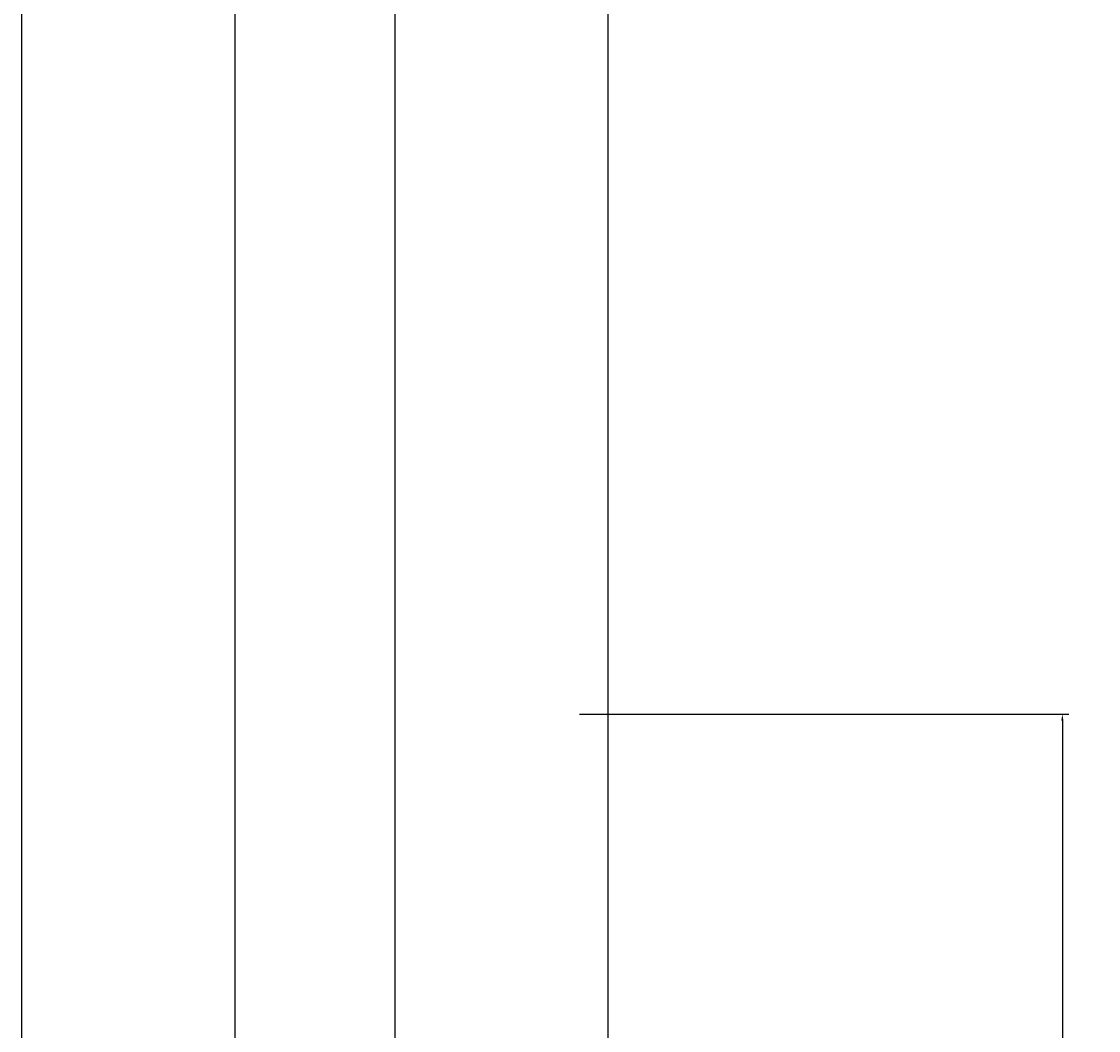
# Model space of a CAD drawing. Units: inches. Extents: x 7359 to 7979, y 33027 to 34263.
# Tile 13 of 32: x 7733 to 7764, y 33417 to 33446. Entities that reach past the tile are written whole.
import ezdxf

# ---------------------------------------------------------------- set-up
doc = ezdxf.new("R2010")
doc.units = ezdxf.units.IN
doc.layers.add('A-ANNO-DIMS', color=2, linetype='Continuous', lineweight=18)
doc.styles.get("Standard").update_dxf_attribs({"font": 'arial.ttf'})
doc.dimstyles.get("Standard").update_dxf_attribs({"dimtxt": 0.18, "dimasz": 0.18, "dimexe": 0.18, "dimexo": 0.0625, "dimgap": 0.09, "dimtad": 0, "dimtih": 1, "dimtoh": 1, "dimdec": 4, "dimzin": 0, "dimdsep": 46, "dimtxsty": 'Standard', "dimcen": 0.09, "dimadec": 0, "dimazin": 0, "dimtfac": 1, "dimtdec": 4, "dimtofl": 0, "dimtmove": 0, "dimatfit": 3, "dimfxl": 1, "dimtolj": 1, "dimtzin": 0, "dimarcsym": 0})

# ---------------------------------------------------------------- blocks, each defined once
blk = doc.blocks.new('*D37')
at = {"layer": 'A-ANNO-DIMS', "color": 0, "lineweight": -2, "transparency": 16777216}
for p, q in [((7748.925, 33426.344), (7762.693, 33426.344)), ((7762.513, 33426.164), (7762.513, 33399.025)), ((7762.513, 33371.524), (7762.513, 33398.662)), ((7748.925, 33371.344), (7762.693, 33371.344))]:
    blk.add_line(p, q, dxfattribs=at)
at = {"layer": 'A-ANNO-DIMS', "color": 0, "transparency": 16777216}
for points in [[(7762.483, 33426.164), (7762.543, 33426.164), (7762.513, 33426.344)], [(7762.483, 33371.524), (7762.543, 33371.524), (7762.513, 33371.344)]]:
    blk.add_solid(points, dxfattribs=at)
at = {"layer": 'Defpoints', "color": 0, "transparency": 16777216}
for p in [(7748.863, 33426.344), (7762.513, 33426.344), (7748.863, 33371.344)]:
    blk.add_point(p, dxfattribs=at)
at = {"layer": 'A-ANNO-DIMS', "color": 0, "transparency": 16777216, "insert": (7762.513, 33398.844), "char_height": 0.18, "attachment_point": 5}
blk.add_mtext('\\A1;55 TYP.', dxfattribs=at)
blk = doc.blocks.new('*D74')
at = {"layer": 'A-ANNO-DIMS', "color": 0, "lineweight": -2, "transparency": 16777216}
for p, q in [((7743.727, 33618.1), (7743.727, 33027.177)), ((7787.034, 33618.1), (7787.034, 33027.177)), ((7743.907, 33027.357), (7765, 33027.357)), ((7786.854, 33027.357), (7765.76, 33027.357))]:
    blk.add_line(p, q, dxfattribs=at)
at = {"layer": 'A-ANNO-DIMS', "color": 0, "transparency": 16777216}
for points in [[(7743.907, 33027.387), (7743.907, 33027.327), (7743.727, 33027.357)], [(7786.854, 33027.387), (7786.854, 33027.327), (7787.034, 33027.357)]]:
    blk.add_solid(points, dxfattribs=at)
at = {"layer": 'Defpoints', "color": 0, "transparency": 16777216}
for p in [(7743.727, 33618.162), (7787.034, 33618.162), (7787.034, 33027.357)]:
    blk.add_point(p, dxfattribs=at)
at = {"layer": 'A-ANNO-DIMS', "color": 0, "transparency": 16777216, "insert": (7765.38, 33027.357), "char_height": 0.18, "attachment_point": 5}
blk.add_mtext('\\A1;43.31', dxfattribs=at)
blk = doc.blocks.new('*D86')
at = {"layer": 'A-ANNO-DIMS', "color": 0, "lineweight": -2, "transparency": 16777216}
for p, q in [((7733.226578, 33475.599789), (7733.226578, 33027.176807)), ((7739.226578, 33475.599789), (7739.226578, 33027.176807)), ((7733.406578, 33027.356807), (7736.077151, 33027.356807)), ((7739.046578, 33027.356807), (7736.376005, 33027.356807))]:
    blk.add_line(p, q, dxfattribs=at)
at = {"layer": 'A-ANNO-DIMS', "color": 0, "transparency": 16777216}
for points in [[(7733.406578, 33027.386807), (7733.406578, 33027.326807), (7733.226578, 33027.356807)], [(7739.046578, 33027.386807), (7739.046578, 33027.326807), (7739.226578, 33027.356807)]]:
    blk.add_solid(points, dxfattribs=at)
at = {"layer": 'Defpoints', "color": 0, "transparency": 16777216}
for p in [(7733.226578, 33475.662289), (7739.226578, 33475.662289), (7739.226578, 33027.356807)]:
    blk.add_point(p, dxfattribs=at)
at = {"layer": 'A-ANNO-DIMS', "color": 0, "transparency": 16777216, "insert": (7736.226578, 33027.356807), "char_height": 0.18, "attachment_point": 5}
blk.add_mtext('\\A1;6', dxfattribs=at)
blk = doc.blocks.new('*D87')
at = {"layer": 'A-ANNO-DIMS', "color": 0, "lineweight": -2, "transparency": 16777216}
for p, q in [((7743.726578, 33453.099789), (7743.726578, 33027.176807)), ((7749.726578, 33453.099789), (7749.726578, 33027.176807)), ((7743.906578, 33027.356807), (7746.577151, 33027.356807)), ((7749.546578, 33027.356807), (7746.876005, 33027.356807))]:
    blk.add_line(p, q, dxfattribs=at)
at = {"layer": 'A-ANNO-DIMS', "color": 0, "transparency": 16777216}
for points in [[(7743.906578, 33027.386807), (7743.906578, 33027.326807), (7743.726578, 33027.356807)], [(7749.546578, 33027.386807), (7749.546578, 33027.326807), (7749.726578, 33027.356807)]]:
    blk.add_solid(points, dxfattribs=at)
at = {"layer": 'Defpoints', "color": 0, "transparency": 16777216}
for p in [(7743.726578, 33453.162289), (7749.726578, 33453.162289), (7749.726578, 33027.356807)]:
    blk.add_point(p, dxfattribs=at)
at = {"layer": 'A-ANNO-DIMS', "color": 0, "transparency": 16777216, "insert": (7746.726578, 33027.356807), "char_height": 0.18, "attachment_point": 5}
blk.add_mtext('\\A1;6', dxfattribs=at)

msp = doc.modelspace()

# ---------------------------------------------------------------- dimensions: what is measured, and where the dimension line sits
at = {"layer": 'A-ANNO-DIMS'}
for base, p1, p2, override, picture, middle in [((7787.0342, 33027.3568), (7743.7266, 33618.1623), (7787.0342, 33618.1623), {"dimdec": 2, "dimlfac": 1, "dimrnd": 0, "dimzin": 0, "dimdsep": 46, "dimlunit": 2}, '*D74', (7765.3804, 33027.3568)), ((7739.2266, 33027.3568), (7733.2266, 33475.6623), (7739.2266, 33475.6623), {"dimdec": 0, "dimlfac": 1, "dimrnd": 0, "dimzin": 0, "dimdsep": 46, "dimlunit": 2}, '*D86', (7736.2266, 33027.3568)), ((7749.7266, 33027.3568), (7743.7266, 33453.1623), (7749.7266, 33453.1623), {"dimdec": 0, "dimlfac": 1, "dimrnd": 0, "dimzin": 0, "dimdsep": 46, "dimlunit": 2}, '*D87', (7746.7266, 33027.3568))]:
    dim = msp.add_linear_dim(base=base, p1=p1, p2=p2, dimstyle='Standard', override=override, dxfattribs=at)
    dim.commit()
    dim.dimension.update_dxf_attribs({"geometry": picture, "text_midpoint": middle})
dim = msp.add_linear_dim(base=(7762.513, 33426.3436), p1=(7748.863, 33371.3436), p2=(7748.863, 33426.3436), angle=90, text='<> TYP.', dimstyle='Standard', override={"dimdec": 0, "dimlfac": 1, "dimrnd": 0, "dimzin": 0, "dimdsep": 46, "dimlunit": 2}, dxfattribs=at)
dim.commit()
dim.dimension.update_dxf_attribs({"geometry": '*D37', "text_midpoint": (7762.513, 33398.8436)})

doc.saveas('drawing.dxf')
